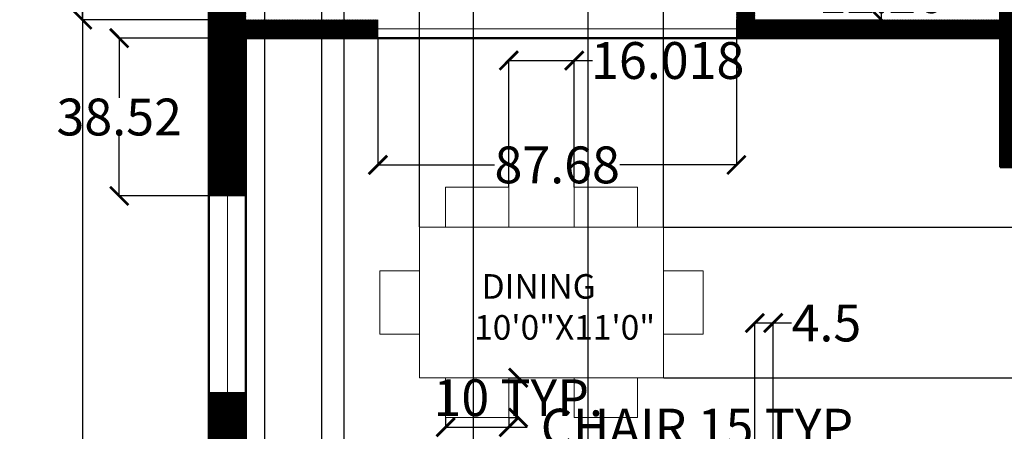
# Model space of a CAD drawing. Units: inches. Extents: x 91 to 526, y 242 to 861.
# Tile 3 of 5: x 91 to 332, y 618 to 719. Entities that reach past the tile are written whole.
import ezdxf

# ---------------------------------------------------------------- set-up
doc = ezdxf.new("R2010")
doc.units = ezdxf.units.IN
doc.header["$MEASUREMENT"] = 0
for name, color, linetype, lineweight in [('A-ANNO-DIMS', 2, 'Continuous', 18), ('A-AREA-IDEN', 7, 'Continuous', 18), ('A-FURN', 8, 'Continuous', 18), ('A-GLAZ', 4, 'Continuous', 18), ('A-WALL', 7, 'Continuous', 50), ('A-WALL-PATT', 252, 'Continuous', 13)]:
    doc.layers.add(name, color=color, linetype=linetype, lineweight=lineweight)
doc.styles.get("Standard").update_dxf_attribs({"font": 'arial.ttf'})
doc.dimstyles.get("Standard").update_dxf_attribs({"dimtxt": 9, "dimasz": 4.5, "dimexe": 0.18, "dimexo": 0.0625, "dimgap": 0.09, "dimtad": 0, "dimtih": 1, "dimtoh": 1, "dimdec": 1, "dimzin": 0, "dimdsep": 46, "dimlunit": 4, "dimtxsty": 'Standard', "dimblk": 'ARCHTICK', "dimcen": 0.09, "dimadec": 0, "dimazin": 0, "dimtfac": 1, "dimtdec": 1, "dimtofl": 0, "dimtmove": 0, "dimatfit": 3, "dimfxl": 1, "dimtolj": 1, "dimtzin": 0, "dimarcsym": 0})

# ---------------------------------------------------------------- blocks, each defined once
blk = doc.blocks.new('WIN-48')
for p, q in [((0, 9), (48, 9)), ((0, 0), (0, 9)), ((48, 9), (48, 0)), ((0, 4.5), (48, 4.5)), ((48, 0), (0, 0))]:
    blk.add_line(p, q)
blk = doc.blocks.new('DINING-CHAIR')
blk.add_lwpolyline([(0, 9.74), (15.43, 9.74), (15.43, 0), (0, 0)], close=True)
blk = doc.blocks.new('_ArchTick')
at = {"color": 0, "linetype": 'ByBlock', "const_width": 0.15}
blk.add_lwpolyline([(-0.5, -0.5), (0.5, 0.5)], dxfattribs=at)
blk = doc.blocks.new('*D13')
at = {"layer": 'A-ANNO-DIMS', "color": 0, "lineweight": -2, "transparency": 16777216}
for p, q in [((195.04, 621.43), (195.04, 619)), ((210.48, 621.43), (210.48, 619)), ((195.04, 619.18), (210.48, 619.18)), ((210.48, 619.18), (214.98, 619.18))]:
    blk.add_line(p, q, dxfattribs=at)
at = {"layer": 'Defpoints', "color": 0, "transparency": 16777216}
for p in [(195.04, 621.5), (210.48, 621.5), (210.48, 619.18)]:
    blk.add_point(p, dxfattribs=at)
at = {"layer": 'A-ANNO-DIMS', "color": 0, "lineweight": -2, "transparency": 16777216, "xscale": 4.5, "yscale": 4.5, "zscale": 4.5, "rotation": 180}
blk.add_blockref('_ArchTick', (195.04, 619.18), dxfattribs=at)
at = {"layer": 'A-ANNO-DIMS', "color": 0, "lineweight": -2, "transparency": 16777216, "xscale": 4.5, "yscale": 4.5, "zscale": 4.5}
blk.add_blockref('_ArchTick', (210.48, 619.18), dxfattribs=at)
at = {"layer": 'A-ANNO-DIMS', "color": 0, "transparency": 16777216, "insert": (258.22, 619.18), "char_height": 9, "attachment_point": 5}
blk.add_mtext('\\A1;CHAIR 15 TYP.', dxfattribs=at)
blk = doc.blocks.new('*D14')
at = {"layer": 'A-ANNO-DIMS', "color": 0, "lineweight": -2, "transparency": 16777216}
for p, q in [((210.54, 631.24), (212.97, 631.24)), ((212.79, 631.24), (212.79, 631.05)), ((210.54, 621.5), (212.97, 621.5)), ((212.79, 621.5), (212.79, 621.68))]:
    blk.add_line(p, q, dxfattribs=at)
at = {"layer": 'Defpoints', "color": 0, "transparency": 16777216}
for p in [(210.48, 631.24), (212.79, 631.24), (210.48, 621.5)]:
    blk.add_point(p, dxfattribs=at)
at = {"layer": 'A-ANNO-DIMS', "color": 0, "lineweight": -2, "transparency": 16777216, "xscale": 4.5, "yscale": 4.5, "zscale": 4.5}
for p, rotation in [((212.79, 631.24), 90), ((212.79, 621.5), 270)]:
    blk.add_blockref('_ArchTick', p, dxfattribs=dict(at, rotation=rotation))
at = {"layer": 'A-ANNO-DIMS', "color": 0, "transparency": 16777216, "insert": (212.79, 626.37), "char_height": 9, "attachment_point": 5}
blk.add_mtext('\\A1;10 TYP.', dxfattribs=at)
blk = doc.blocks.new('*D18')
at = {"layer": 'A-ANNO-DIMS', "color": 0, "lineweight": -2, "transparency": 16777216}
for p, q in [((137.1, 823.67), (106.03, 823.67)), ((106.21, 823.67), (106.21, 570.36)), ((106.21, 307.67), (106.21, 560.99)), ((137.1, 307.67), (106.03, 307.67))]:
    blk.add_line(p, q, dxfattribs=at)
at = {"layer": 'Defpoints', "color": 0, "transparency": 16777216}
for p in [(106.21, 823.67), (137.16, 823.67), (137.16, 307.67)]:
    blk.add_point(p, dxfattribs=at)
at = {"layer": 'A-ANNO-DIMS', "color": 0, "lineweight": -2, "transparency": 16777216, "xscale": 4.5, "yscale": 4.5, "zscale": 4.5}
for p, rotation in [((106.21, 823.67), 90), ((106.21, 307.67), 270)]:
    blk.add_blockref('_ArchTick', p, dxfattribs=dict(at, rotation=rotation))
at = {"layer": 'A-ANNO-DIMS', "color": 0, "transparency": 16777216, "insert": (106.21, 565.67), "char_height": 9, "attachment_point": 5}
blk.add_mtext('\\A1;516', dxfattribs=at)
blk = doc.blocks.new('*D28')
at = {"layer": 'A-ANNO-DIMS', "color": 0, "lineweight": -2, "transparency": 16777216}
for p, q in [((146.1, 714.17), (115.03, 714.17)), ((115.21, 714.17), (115.21, 699.6)), ((115.21, 675.65), (115.21, 690.22)), ((146.1, 675.65), (115.03, 675.65))]:
    blk.add_line(p, q, dxfattribs=at)
at = {"layer": 'Defpoints', "color": 0, "transparency": 16777216}
for p in [(115.21, 714.17), (146.16, 714.17), (146.16, 675.65)]:
    blk.add_point(p, dxfattribs=at)
at = {"layer": 'A-ANNO-DIMS', "color": 0, "lineweight": -2, "transparency": 16777216, "xscale": 4.5, "yscale": 4.5, "zscale": 4.5}
for p, rotation in [((115.21, 714.17), 90), ((115.21, 675.65), 270)]:
    blk.add_blockref('_ArchTick', p, dxfattribs=dict(at, rotation=rotation))
at = {"layer": 'A-ANNO-DIMS', "color": 0, "transparency": 16777216, "insert": (115.21, 694.91), "char_height": 9, "attachment_point": 5}
blk.add_mtext('\\A1;38.52', dxfattribs=at)
blk = doc.blocks.new('*D36')
at = {"layer": 'A-ANNO-DIMS', "color": 0, "lineweight": -2, "transparency": 16777216}
for p, q in [((270.66, 613.73), (270.66, 644.8)), ((270.66, 644.62), (275.16, 644.62)), ((275.16, 613.73), (275.16, 644.8)), ((275.16, 644.62), (279.66, 644.62))]:
    blk.add_line(p, q, dxfattribs=at)
at = {"layer": 'Defpoints', "color": 0, "transparency": 16777216}
for p in [(275.16, 644.62), (270.66, 613.67), (275.16, 613.67)]:
    blk.add_point(p, dxfattribs=at)
at = {"layer": 'A-ANNO-DIMS', "color": 0, "lineweight": -2, "transparency": 16777216, "xscale": 4.5, "yscale": 4.5, "zscale": 4.5, "rotation": 180}
blk.add_blockref('_ArchTick', (270.66, 644.62), dxfattribs=at)
at = {"layer": 'A-ANNO-DIMS', "color": 0, "lineweight": -2, "transparency": 16777216, "xscale": 4.5, "yscale": 4.5, "zscale": 4.5}
blk.add_blockref('_ArchTick', (275.16, 644.62), dxfattribs=at)
at = {"layer": 'A-ANNO-DIMS', "color": 0, "transparency": 16777216, "insert": (288.16, 644.62), "char_height": 9, "attachment_point": 5}
blk.add_mtext('\\A1;4.5', dxfattribs=at)
blk = doc.blocks.new('*D37')
at = {"layer": 'A-ANNO-DIMS', "color": 0, "lineweight": -2, "transparency": 16777216}
for p, q in [((178.48, 714.11), (178.48, 683.04)), ((266.16, 714.11), (266.16, 683.04)), ((178.48, 683.22), (207.03, 683.22)), ((266.16, 683.22), (237.61, 683.22))]:
    blk.add_line(p, q, dxfattribs=at)
at = {"layer": 'Defpoints', "color": 0, "transparency": 16777216}
for p in [(178.48, 714.17), (266.16, 714.17), (178.48, 683.22)]:
    blk.add_point(p, dxfattribs=at)
at = {"layer": 'A-ANNO-DIMS', "color": 0, "lineweight": -2, "transparency": 16777216, "xscale": 4.5, "yscale": 4.5, "zscale": 4.5}
for p, rotation in [((178.48, 683.22), 179.9999999999999), ((266.16, 683.22), 359.9999999999999)]:
    blk.add_blockref('_ArchTick', p, dxfattribs=dict(at, rotation=rotation))
at = {"layer": 'A-ANNO-DIMS', "color": 0, "transparency": 16777216, "insert": (222.32, 683.22), "char_height": 9, "attachment_point": 5}
blk.add_mtext('\\A1;87.68', dxfattribs=at)
blk = doc.blocks.new('*D38')
at = {"layer": 'A-ANNO-DIMS', "color": 0, "lineweight": -2, "transparency": 16777216}
for p, q in [((146.16, 718.61), (146.16, 276.54)), ((170.16, 718.61), (170.16, 276.54)), ((146.16, 276.72), (151.57, 276.72)), ((170.16, 276.72), (164.75, 276.72))]:
    blk.add_line(p, q, dxfattribs=at)
at = {"layer": 'Defpoints', "color": 0, "transparency": 16777216}
for p in [(146.16, 718.67), (170.16, 718.67), (170.16, 276.72)]:
    blk.add_point(p, dxfattribs=at)
at = {"layer": 'A-ANNO-DIMS', "color": 0, "lineweight": -2, "transparency": 16777216, "xscale": 4.5, "yscale": 4.5, "zscale": 4.5, "rotation": 180}
blk.add_blockref('_ArchTick', (146.16, 276.72), dxfattribs=at)
at = {"layer": 'A-ANNO-DIMS', "color": 0, "lineweight": -2, "transparency": 16777216, "xscale": 4.5, "yscale": 4.5, "zscale": 4.5}
blk.add_blockref('_ArchTick', (170.16, 276.72), dxfattribs=at)
at = {"layer": 'A-ANNO-DIMS', "color": 0, "transparency": 16777216, "insert": (158.16, 276.72), "char_height": 9, "attachment_point": 5}
blk.add_mtext('\\A1;24', dxfattribs=at)
blk = doc.blocks.new('*D39')
at = {"layer": 'A-ANNO-DIMS', "color": 0, "lineweight": -2, "transparency": 16777216}
for p, q in [((201.78, 794.78), (201.78, 276.54)), ((229.79, 794.78), (229.79, 276.54)), ((201.78, 276.72), (229.79, 276.72)), ((229.79, 276.72), (234.29, 276.72))]:
    blk.add_line(p, q, dxfattribs=at)
at = {"layer": 'Defpoints', "color": 0, "transparency": 16777216}
for p in [(201.78, 794.84), (229.79, 794.84), (229.79, 276.72)]:
    blk.add_point(p, dxfattribs=at)
at = {"layer": 'A-ANNO-DIMS', "color": 0, "lineweight": -2, "transparency": 16777216, "xscale": 4.5, "yscale": 4.5, "zscale": 4.5, "rotation": 180}
blk.add_blockref('_ArchTick', (201.78, 276.72), dxfattribs=at)
at = {"layer": 'A-ANNO-DIMS', "color": 0, "lineweight": -2, "transparency": 16777216, "xscale": 4.5, "yscale": 4.5, "zscale": 4.5}
blk.add_blockref('_ArchTick', (229.79, 276.72), dxfattribs=at)
at = {"layer": 'A-ANNO-DIMS', "color": 0, "transparency": 16777216, "insert": (248.77, 276.72), "char_height": 9, "attachment_point": 5}
blk.add_mtext('\\A1;28.01', dxfattribs=at)
blk = doc.blocks.new('*D41')
at = {"layer": 'A-ANNO-DIMS', "color": 0, "lineweight": -2, "transparency": 16777216}
for p, q in [((150.78, 748.14), (150.78, 276.54)), ((164.66, 748.14), (164.66, 276.54)), ((150.78, 276.72), (164.66, 276.72)), ((164.66, 276.72), (169.16, 276.72))]:
    blk.add_line(p, q, dxfattribs=at)
at = {"layer": 'Defpoints', "color": 0, "transparency": 16777216}
for p in [(150.78, 748.2), (164.66, 748.2), (164.66, 276.72)]:
    blk.add_point(p, dxfattribs=at)
at = {"layer": 'A-ANNO-DIMS', "color": 0, "lineweight": -2, "transparency": 16777216, "xscale": 4.5, "yscale": 4.5, "zscale": 4.5, "rotation": 180}
blk.add_blockref('_ArchTick', (150.78, 276.72), dxfattribs=at)
at = {"layer": 'A-ANNO-DIMS', "color": 0, "lineweight": -2, "transparency": 16777216, "xscale": 4.5, "yscale": 4.5, "zscale": 4.5}
blk.add_blockref('_ArchTick', (164.66, 276.72), dxfattribs=at)
at = {"layer": 'A-ANNO-DIMS', "color": 0, "transparency": 16777216, "insert": (184.01, 276.72), "char_height": 9, "attachment_point": 5}
blk.add_mtext('\\A1;13.87', dxfattribs=at)
blk = doc.blocks.new('*D43')
at = {"layer": 'A-ANNO-DIMS', "color": 0, "lineweight": -2, "transparency": 16777216}
for p, q in [((150.72, 748.2), (106.03, 748.2)), ((106.21, 748.2), (106.21, 738.12)), ((106.21, 718.67), (106.21, 728.75)), ((146.1, 718.67), (106.03, 718.67))]:
    blk.add_line(p, q, dxfattribs=at)
at = {"layer": 'Defpoints', "color": 0, "transparency": 16777216}
for p in [(106.21, 748.2), (150.78, 748.2), (146.16, 718.67)]:
    blk.add_point(p, dxfattribs=at)
at = {"layer": 'A-ANNO-DIMS', "color": 0, "lineweight": -2, "transparency": 16777216, "xscale": 4.5, "yscale": 4.5, "zscale": 4.5}
for p, rotation in [((106.21, 748.2), 90), ((106.21, 718.67), 270)]:
    blk.add_blockref('_ArchTick', p, dxfattribs=dict(at, rotation=rotation))
at = {"layer": 'A-ANNO-DIMS', "color": 0, "transparency": 16777216, "insert": (106.21, 733.44), "char_height": 9, "attachment_point": 5}
blk.add_mtext('\\A1;29.53', dxfattribs=at)
blk = doc.blocks.new('*D44')
at = {"layer": 'A-ANNO-DIMS', "color": 0, "lineweight": -2, "transparency": 16777216}
for p, q in [((201.78, 794.78), (201.78, 276.54)), ((170.16, 790.61), (170.16, 276.54)), ((170.16, 276.72), (170.74, 276.72)), ((201.78, 276.72), (201.2, 276.72))]:
    blk.add_line(p, q, dxfattribs=at)
at = {"layer": 'Defpoints', "color": 0, "transparency": 16777216}
for p in [(201.78, 794.84), (170.16, 790.67), (201.78, 276.72)]:
    blk.add_point(p, dxfattribs=at)
at = {"layer": 'A-ANNO-DIMS', "color": 0, "lineweight": -2, "transparency": 16777216, "xscale": 4.5, "yscale": 4.5, "zscale": 4.5, "rotation": 180}
blk.add_blockref('_ArchTick', (170.16, 276.72), dxfattribs=at)
at = {"layer": 'A-ANNO-DIMS', "color": 0, "lineweight": -2, "transparency": 16777216, "xscale": 4.5, "yscale": 4.5, "zscale": 4.5}
blk.add_blockref('_ArchTick', (201.78, 276.72), dxfattribs=at)
at = {"layer": 'A-ANNO-DIMS', "color": 0, "transparency": 16777216, "insert": (185.97, 276.72), "char_height": 9, "attachment_point": 5}
blk.add_mtext('\\A1;31.62', dxfattribs=at)
blk = doc.blocks.new('*D45')
at = {"layer": 'A-ANNO-DIMS', "color": 0, "lineweight": -2, "transparency": 16777216}
for p, q in [((188.65, 668.08), (188.65, 854.8)), ((188.65, 854.62), (203.21, 854.62)), ((248.32, 854.62), (233.76, 854.62)), ((248.32, 668.08), (248.32, 854.8))]:
    blk.add_line(p, q, dxfattribs=at)
at = {"layer": 'Defpoints', "color": 0, "transparency": 16777216}
for p in [(248.32, 854.62), (188.65, 668.02), (248.32, 668.02)]:
    blk.add_point(p, dxfattribs=at)
at = {"layer": 'A-ANNO-DIMS', "color": 0, "lineweight": -2, "transparency": 16777216, "xscale": 4.5, "yscale": 4.5, "zscale": 4.5, "rotation": 180}
blk.add_blockref('_ArchTick', (188.65, 854.62), dxfattribs=at)
at = {"layer": 'A-ANNO-DIMS', "color": 0, "lineweight": -2, "transparency": 16777216, "xscale": 4.5, "yscale": 4.5, "zscale": 4.5}
blk.add_blockref('_ArchTick', (248.32, 854.62), dxfattribs=at)
at = {"layer": 'A-ANNO-DIMS', "color": 0, "transparency": 16777216, "insert": (218.48, 854.62), "char_height": 9, "attachment_point": 5}
blk.add_mtext('\\A1;59.66', dxfattribs=at)
blk = doc.blocks.new('*D46')
at = {"layer": 'A-ANNO-DIMS', "color": 0, "lineweight": -2, "transparency": 16777216}
for p, q in [((248.38, 668.02), (507.29, 668.02)), ((507.11, 668.02), (507.11, 654.31)), ((507.11, 631.24), (507.11, 644.94)), ((248.38, 631.24), (507.29, 631.24))]:
    blk.add_line(p, q, dxfattribs=at)
at = {"layer": 'Defpoints', "color": 0, "transparency": 16777216}
for p in [(248.32, 668.02), (507.11, 668.02), (248.32, 631.24)]:
    blk.add_point(p, dxfattribs=at)
at = {"layer": 'A-ANNO-DIMS', "color": 0, "lineweight": -2, "transparency": 16777216, "xscale": 4.5, "yscale": 4.5, "zscale": 4.5}
for p, rotation in [((507.11, 668.02), 90), ((507.11, 631.24), 270)]:
    blk.add_blockref('_ArchTick', p, dxfattribs=dict(at, rotation=rotation))
at = {"layer": 'A-ANNO-DIMS', "color": 0, "transparency": 16777216, "insert": (507.11, 649.63), "char_height": 9, "attachment_point": 5}
blk.add_mtext('\\A1;36.78', dxfattribs=at)
blk = doc.blocks.new('*D47')
at = {"layer": 'A-ANNO-DIMS', "color": 0, "lineweight": -2, "transparency": 16777216}
for p, q in [((210.48, 677.82), (210.48, 708.89)), ((210.48, 708.71), (226.49, 708.71)), ((226.49, 677.82), (226.49, 708.89)), ((226.49, 708.71), (230.99, 708.71))]:
    blk.add_line(p, q, dxfattribs=at)
at = {"layer": 'Defpoints', "color": 0, "transparency": 16777216}
for p in [(226.49, 708.71), (210.48, 677.76), (226.49, 677.76)]:
    blk.add_point(p, dxfattribs=at)
at = {"layer": 'A-ANNO-DIMS', "color": 0, "lineweight": -2, "transparency": 16777216, "xscale": 4.5, "yscale": 4.5, "zscale": 4.5, "rotation": 180}
blk.add_blockref('_ArchTick', (210.48, 708.71), dxfattribs=at)
at = {"layer": 'A-ANNO-DIMS', "color": 0, "lineweight": -2, "transparency": 16777216, "xscale": 4.5, "yscale": 4.5, "zscale": 4.5}
blk.add_blockref('_ArchTick', (226.49, 708.71), dxfattribs=at)
at = {"layer": 'A-ANNO-DIMS', "color": 0, "transparency": 16777216, "insert": (249.35, 708.71), "char_height": 9, "attachment_point": 5}
blk.add_mtext('\\A1;16.018', dxfattribs=at)
blk = doc.blocks.new('*D54')
at = {"layer": 'A-ANNO-DIMS', "color": 0, "lineweight": -2, "transparency": 16777216}
for p, q in [((270.72, 730.93), (301.79, 730.93)), ((301.61, 730.93), (301.61, 729.49)), ((301.61, 718.67), (301.61, 720.12)), ((270.72, 718.67), (301.79, 718.67))]:
    blk.add_line(p, q, dxfattribs=at)
at = {"layer": 'Defpoints', "color": 0, "transparency": 16777216}
for p in [(270.66, 730.93), (270.66, 718.67), (301.61, 718.67)]:
    blk.add_point(p, dxfattribs=at)
at = {"layer": 'A-ANNO-DIMS', "color": 0, "lineweight": -2, "transparency": 16777216, "xscale": 4.5, "yscale": 4.5, "zscale": 4.5}
for p, rotation in [((301.61, 730.93), 90), ((301.61, 718.67), 270)]:
    blk.add_blockref('_ArchTick', p, dxfattribs=dict(at, rotation=rotation))
at = {"layer": 'A-ANNO-DIMS', "color": 0, "transparency": 16777216, "insert": (301.61, 724.8), "char_height": 9, "attachment_point": 5}
blk.add_mtext('\\A1;12.26', dxfattribs=at)

msp = doc.modelspace()

# ---------------------------------------------------------------- hatches: boundary and pattern name
at = {"layer": 'A-WALL-PATT'}
h = msp.add_hatch(dxfattribs=at)
h.set_pattern_fill('ANSI31', color=256)
h.paths.add_polyline_path([(476.1605, 544.131), (467.1605, 544.131), (467.1605, 469.6714), (381.2784, 469.6714), (381.2784, 467.1295, -0.01443214), (381.4527, 465.1714), (467.1605, 465.1714), (467.1605, 417.4774), (476.1605, 417.4774)])
h.paths.add_polyline_path([(476.1605, 637.294), (467.1605, 637.294), (467.1605, 618.1714), (383.1605, 618.1714), (383.1605, 650.6481), (381.8098, 650.6481, -0.04281846), (378.6605, 650.378), (378.6605, 618.1714), (378.6605, 613.6714), (467.1605, 613.6714), (467.1605, 592.131), (476.1605, 592.131)])
h.paths.add_polyline_path([(476.1605, 699.6337), (467.1605, 699.6337), (467.1605, 682.6714), (378.6605, 682.6714), (367.8126, 682.6714), (367.8126, 678.1714), (378.6605, 678.1714), (378.6605, 668.8665), (383.1605, 668.8665), (383.1605, 678.1714), (467.1605, 678.1714), (467.1605, 661.294), (476.1605, 661.294)])
h.paths.add_polyline_path([(476.1605, 823.6714), (423.2305, 823.6714), (423.2305, 814.6714), (467.1605, 814.6714), (467.1605, 747.6337), (476.1605, 747.6337)])
h.paths.add_polyline_path([(375.2305, 823.6714), (311.1029, 823.6714), (311.1029, 814.6714), (330.6605, 814.6714), (330.6605, 682.6714), (335.1605, 682.6714), (335.1605, 814.6714), (375.2305, 814.6714)])
h.paths.add_polyline_path([(287.1029, 823.6714), (230.7133, 823.6714), (230.7133, 814.6714), (266.1605, 814.6714), (266.1605, 755.4247), (270.6605, 755.4247), (270.6605, 814.6714), (287.1029, 814.6714)])
h.paths.add_polyline_path([(182.7133, 823.6714), (137.1605, 823.6714), (137.1605, 675.6513), (146.1605, 675.6513), (146.1605, 714.1714), (178.4758, 714.1714), (178.4758, 718.6714), (146.1605, 718.6714), (146.1605, 814.6714), (182.7133, 814.6714)])
h.paths.add_polyline_path([(146.1605, 577.6714), (206.1605, 577.6714), (206.1605, 557.5953), (210.6605, 557.5953), (210.6605, 577.6714), (233.4933, 577.6714), (233.4933, 582.1714), (210.6605, 582.1714), (146.1605, 582.1714), (146.1605, 627.6513), (137.1605, 627.6513), (137.1605, 508.0167), (146.1605, 508.0167), (146.1605, 525.1714), (210.6605, 525.1714), (233.4933, 525.1714), (233.4933, 529.6714), (210.6605, 529.6714), (210.6605, 536.5826), (206.1605, 536.5826), (206.1605, 529.6714), (146.1605, 529.6714)])
h.paths.add_polyline_path([(146.1605, 460.0167), (137.1605, 460.0167), (137.1605, 360.2935), (146.1605, 360.2935), (146.1605, 376.6714), (210.6605, 376.6714), (213.2441, 376.6714, -0.02418169), (213.3544, 378.9513), (213.3544, 381.1714), (210.6605, 381.1714), (146.1605, 381.1714)])
h.paths.add_polyline_path([(146.1605, 336.2935), (137.1605, 336.2935), (137.1605, 307.6714), (146.1605, 307.6714), (177.3362, 307.6714), (177.3362, 316.6714), (146.1605, 316.6714)])
h.paths.add_polyline_path([(393.6086, 316.6714), (323.4726, 316.6714), (323.4726, 307.6714), (393.6086, 307.6714)])
h.paths.add_polyline_path([(256.39, 316.6714), (201.3362, 316.6714), (201.3362, 307.6714), (256.39, 307.6714)])
h.paths.add_polyline_path([(246.6605, 376.6714), (246.6605, 381.1714), (236.8559, 381.1714), (236.8559, 376.6714), (242.1605, 376.6714), (242.1605, 316.6714), (246.6605, 316.6714)])
h = msp.add_hatch(dxfattribs=at)
h.set_pattern_fill('ANSI31', color=256)
h.paths.add_polyline_path([(476.1605, 369.4774), (467.1605, 369.4774), (467.1605, 316.6714), (417.6086, 316.6714), (417.6086, 307.6714), (476.1605, 307.6714)])
h.paths.add_polyline_path([(330.6605, 718.6714), (270.6605, 718.6714), (270.6605, 730.9304), (266.1605, 730.9304), (266.1605, 718.6714), (266.1605, 714.1714), (270.6605, 714.1714), (330.6605, 714.1714)])

# ---------------------------------------------------------------- linework, layer by layer
at = {"layer": 'A-FURN'}
for p, q in [((188.6533, 668.0163), (248.3166, 668.0163)), ((188.6533, 631.2365), (188.6533, 668.0163)), ((248.3166, 668.0163), (248.3166, 631.2365)), ((248.3166, 631.2365), (188.6533, 631.2365))]:
    msp.add_line(p, q, dxfattribs=at)
at = {"layer": 'A-GLAZ'}
for p, q in [((178.4758, 718.6714), (178.4758, 714.1714)), ((266.1605, 718.6714), (266.1605, 714.1714)), ((178.4758, 716.4214), (266.1605, 716.4214))]:
    msp.add_line(p, q, dxfattribs=at)
at = {"layer": 'A-WALL'}
for p, q in [((137.1605, 823.6714), (137.1605, 307.6714)), ((330.6605, 814.6714), (330.6605, 682.6714)), ((146.1605, 714.1714), (266.1605, 714.1714)), ((146.1605, 714.1714), (146.1605, 582.1714)), ((270.6605, 714.1714), (266.1605, 714.1714)), ((270.6605, 714.1714), (330.6605, 714.1714)), ((335.1605, 682.6714), (330.6605, 682.6714))]:
    msp.add_line(p, q, dxfattribs=at)

# ---------------------------------------------------------------- block references
at = {"layer": 'A-FURN', "extrusion": (0, 0, -1), "zscale": -1}
for p, rotation in [((-195.042, 677.7558), 180), ((-188.6535, 657.3432), 270.0000000000006)]:
    msp.add_blockref('DINING-CHAIR', p, dxfattribs=dict(at, rotation=rotation))
at = {"layer": 'A-FURN'}
for p, rotation in [((241.928, 677.7558), 180), ((248.3165, 657.3432), 270.0000000000008)]:
    msp.add_blockref('DINING-CHAIR', p, dxfattribs=dict(at, rotation=rotation))
msp.add_blockref('DINING-CHAIR', (195.042, 621.497), dxfattribs=at)
at = {"layer": 'A-FURN', "extrusion": (0, 0, -1), "zscale": -1}
msp.add_blockref('DINING-CHAIR', (-241.928, 621.497), dxfattribs=at)
at = {"layer": 'A-GLAZ', "rotation": 270.0000000000002}
msp.add_blockref('WIN-48', (137.1601, 675.6516), dxfattribs=at)

# ---------------------------------------------------------------- texts
at = {"layer": 'A-AREA-IDEN', "insert": (200.181, 656.5399), "char_height": 6, "attachment_point": 1}
msp.add_mtext_dynamic_manual_height_columns('  DINING\\P 10\'0"X11\'0"', width=356.121763, gutter_width=1, heights=[0], dxfattribs=at)

# ---------------------------------------------------------------- dimensions: what is measured, and where the dimension line sits
at = {"layer": 'A-ANNO-DIMS'}
for base, p1, p2, override, picture, middle in [((248.3166, 854.6214), (188.6533, 668.0163), (248.3166, 668.0163), {"dimdec": 2, "dimlfac": 1, "dimrnd": 0, "dimzin": 0, "dimdsep": 46, "dimlunit": 2}, '*D45', (218.485, 854.6214)), ((201.7777, 276.7214), (170.1605, 790.6714), (201.7777, 794.8389), {"dimdec": 2, "dimlfac": 1, "dimrnd": 0, "dimzin": 0, "dimdsep": 46, "dimlunit": 2}, '*D44', (185.9691, 276.7214)), ((229.7885, 276.7214), (201.7777, 794.8389), (229.7885, 794.8389), {"dimdec": 2, "dimlfac": 1, "dimrnd": 0, "dimzin": 0, "dimdsep": 46, "dimlunit": 2}, '*D39', (248.7718, 276.7214)), ((164.6554, 276.7214), (150.7847, 748.2001), (164.6554, 748.2001), {"dimdec": 2, "dimlfac": 1, "dimrnd": 0, "dimzin": 0, "dimdsep": 46, "dimlunit": 2}, '*D41', (184.007, 276.7214)), ((170.1605, 276.7214), (146.1605, 718.6714), (170.1605, 718.6714), {"dimdec": 0, "dimlfac": 1, "dimrnd": 0, "dimzin": 0, "dimdsep": 46, "dimlunit": 2}, '*D38', (158.1605, 276.7214)), ((226.4941, 708.7056), (210.4759, 677.7556), (226.4941, 677.7556), {"dimdec": 3, "dimlfac": 1, "dimrnd": 0, "dimzin": 0, "dimdsep": 46, "dimlunit": 2}, '*D47', (249.3511, 708.7056)), ((275.1605, 644.6214), (270.6605, 613.6714), (275.1605, 613.6714), {"dimdec": 1, "dimlfac": 1, "dimrnd": 0, "dimzin": 0, "dimdsep": 46, "dimlunit": 2}, '*D36', (288.1581, 644.6214))]:
    dim = msp.add_linear_dim(base=base, p1=p1, p2=p2, dimstyle='Standard', override=override, dxfattribs=at)
    dim.commit()
    dim.dimension.update_dxf_attribs({"geometry": picture, "text_midpoint": middle})
for base, p1, p2, angle, override, picture, middle in [((106.2105, 823.6714), (137.1605, 307.6714), (137.1605, 823.6714), 90, {"dimdec": 0, "dimlfac": 1, "dimrnd": 0, "dimzin": 0, "dimdsep": 46, "dimlunit": 2}, '*D18', (106.2105, 565.6714)), ((106.2105, 748.2001), (146.1605, 718.6714), (150.7847, 748.2001), 90, {"dimdec": 2, "dimlfac": 1, "dimrnd": 0, "dimzin": 0, "dimdsep": 46, "dimlunit": 2}, '*D43', (106.2105, 733.4358)), ((301.6105, 718.6714), (270.6605, 730.9304), (270.6605, 718.6714), 270, {"dimdec": 2, "dimlfac": 1, "dimrnd": 0, "dimzin": 0, "dimdsep": 46, "dimlunit": 2}, '*D54', (301.6105, 724.8009)), ((115.2105, 714.1714), (146.1605, 675.6513), (146.1605, 714.1714), 90, {"dimdec": 2, "dimlfac": 1, "dimrnd": 0, "dimzin": 0, "dimdsep": 46, "dimlunit": 2}, '*D28', (115.2105, 694.9114)), ((178.4758, 683.2214), (266.1605, 714.1714), (178.4758, 714.1714), 180, {"dimdec": 2, "dimlfac": 1, "dimrnd": 0, "dimzin": 0, "dimdsep": 46, "dimlunit": 2}, '*D37', (222.3182, 683.2214)), ((507.1105, 668.0163), (248.3166, 631.2365), (248.3166, 668.0163), 90, {"dimdec": 2, "dimlfac": 1, "dimrnd": 0, "dimzin": 0, "dimdsep": 46, "dimlunit": 2}, '*D46', (507.1105, 649.6264))]:
    dim = msp.add_linear_dim(base=base, p1=p1, p2=p2, angle=angle, dimstyle='Standard', override=override, dxfattribs=at)
    dim.commit()
    dim.dimension.update_dxf_attribs({"geometry": picture, "text_midpoint": middle})
dim = msp.add_linear_dim(base=(210.4759, 619.182), p1=(195.0418, 621.4971), p2=(210.4759, 621.4971), text='CHAIR <> TYP.', dimstyle='Standard', override={"dimdec": 0, "dimlfac": 1, "dimrnd": 0, "dimzin": 0, "dimdsep": 46, "dimlunit": 2}, dxfattribs=at)
dim.commit()
dim.dimension.update_dxf_attribs({"geometry": '*D13', "text_midpoint": (258.2241, 619.182)})
dim = msp.add_linear_dim(base=(212.791, 631.2365), p1=(210.4759, 621.4971), p2=(210.4759, 631.2365), angle=90, text='<> TYP.', dimstyle='Standard', override={"dimdec": 0, "dimlfac": 1, "dimrnd": 0, "dimzin": 0, "dimdsep": 46, "dimlunit": 2}, dxfattribs=at)
dim.commit()
dim.dimension.update_dxf_attribs({"geometry": '*D14', "text_midpoint": (212.791, 626.3668)})

doc.saveas('drawing.dxf')
